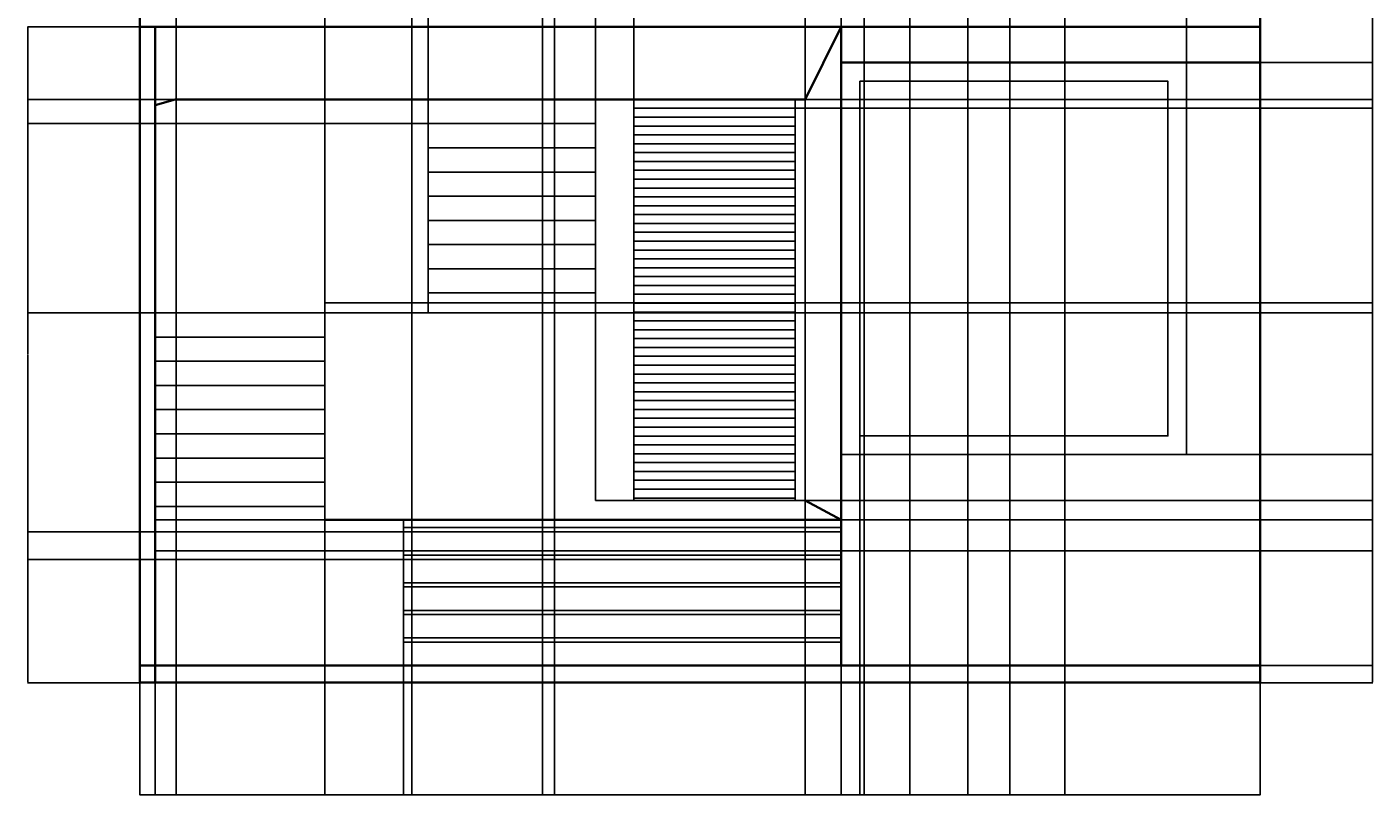
# Model space of a CAD drawing. Units: feet. Extents: x 2373 to 3800, y 799 to 1842.
# Tile 2 of 4: x 3224 to 3800, y 799 to 1129. Entities that reach past the tile are written whole.
import ezdxf

# ---------------------------------------------------------------- set-up
doc = ezdxf.new("R2010")
doc.units = ezdxf.units.FT
for name, color, linetype, lineweight in [('A-ANNO-DIMS', 2, 'Continuous', 18), ('A-DOOR', 4, 'Continuous', 25), ('A-ELEV', 7, 'Continuous', 35), ('A-FLOR-STRS', 3, 'Continuous', 25), ('A-GLAZ', 4, 'Continuous', 25)]:
    doc.layers.add(name, color=color, linetype=linetype, lineweight=lineweight)
doc.styles.get("Standard").update_dxf_attribs({"font": 'arial.ttf'})
doc.dimstyles.get("Standard").update_dxf_attribs({"dimtxt": 0.18, "dimasz": 0.18, "dimexe": 0.18, "dimexo": 0.0625, "dimgap": 0.09, "dimtad": 0, "dimtih": 1, "dimtoh": 1, "dimdec": 1, "dimzin": 0, "dimdsep": 46, "dimlunit": 3, "dimtxsty": 'Standard', "dimcen": 0.09, "dimadec": 0, "dimazin": 0, "dimtfac": 1, "dimtdec": 1, "dimtofl": 0, "dimtmove": 0, "dimatfit": 3, "dimfxl": 1, "dimtolj": 1, "dimtzin": 0, "dimarcsym": 0})

# ---------------------------------------------------------------- blocks, each defined once
blk = doc.blocks.new('*D7')
at = {"layer": 'A-ANNO-DIMS', "color": 0, "lineweight": -2, "transparency": 16777216}
for p, q in [((3271.99, 847.59), (3271.99, 799.47)), ((3751.99, 847.59), (3751.99, 799.47)), ((3272.17, 799.65), (3511.69, 799.65)), ((3751.81, 799.65), (3512.28, 799.65))]:
    blk.add_line(p, q, dxfattribs=at)
at = {"layer": 'A-ANNO-DIMS', "color": 0, "transparency": 16777216}
for points in [[(3272.17, 799.68), (3272.17, 799.62), (3271.99, 799.65)], [(3751.81, 799.68), (3751.81, 799.62), (3751.99, 799.65)]]:
    blk.add_solid(points, dxfattribs=at)
at = {"layer": 'Defpoints', "color": 0, "transparency": 16777216}
for p in [(3271.99, 847.65), (3751.99, 847.65), (3751.99, 799.65)]:
    blk.add_point(p, dxfattribs=at)
at = {"layer": 'A-ANNO-DIMS', "color": 0, "transparency": 16777216, "insert": (3511.99, 799.65), "char_height": 0.18, "attachment_point": 5}
blk.add_mtext('\\A1;480', dxfattribs=at)
blk = doc.blocks.new('*D8')
at = {"layer": 'A-ANNO-DIMS', "color": 0, "lineweight": -2, "transparency": 16777216}
for p, q in [((3752.05, 1793.54), (3800.17, 1793.54)), ((3799.99, 1793.36), (3799.99, 1320.78)), ((3799.99, 847.83), (3799.99, 1320.41)), ((3752.05, 847.65), (3800.17, 847.65))]:
    blk.add_line(p, q, dxfattribs=at)
at = {"layer": 'A-ANNO-DIMS', "color": 0, "transparency": 16777216}
for points in [[(3799.96, 1793.36), (3800.02, 1793.36), (3799.99, 1793.54)], [(3799.96, 847.83), (3800.02, 847.83), (3799.99, 847.65)]]:
    blk.add_solid(points, dxfattribs=at)
at = {"layer": 'Defpoints', "color": 0, "transparency": 16777216}
for p in [(3751.99, 1793.54), (3799.99, 1793.54), (3751.99, 847.65)]:
    blk.add_point(p, dxfattribs=at)
at = {"layer": 'A-ANNO-DIMS', "color": 0, "transparency": 16777216, "insert": (3799.99, 1320.6), "char_height": 0.18, "attachment_point": 5}
blk.add_mtext('\\A1;945.9', dxfattribs=at)
blk = doc.blocks.new('*D9')
at = {"layer": 'A-ANNO-DIMS', "color": 0, "lineweight": -2, "transparency": 16777216}
for p, q in [((3271.92, 1128.67), (3223.81, 1128.67)), ((3223.99, 1128.49), (3223.99, 988.34)), ((3223.99, 847.83), (3223.99, 987.98)), ((3271.92, 847.65), (3223.81, 847.65))]:
    blk.add_line(p, q, dxfattribs=at)
at = {"layer": 'A-ANNO-DIMS', "color": 0, "transparency": 16777216}
for points in [[(3223.96, 1128.49), (3224.02, 1128.49), (3223.99, 1128.67)], [(3223.96, 847.83), (3224.02, 847.83), (3223.99, 847.65)]]:
    blk.add_solid(points, dxfattribs=at)
at = {"layer": 'Defpoints', "color": 0, "transparency": 16777216}
for p in [(3223.99, 1128.67), (3271.99, 1128.67), (3271.99, 847.65)]:
    blk.add_point(p, dxfattribs=at)
at = {"layer": 'A-ANNO-DIMS', "color": 0, "transparency": 16777216, "insert": (3223.99, 988.16), "char_height": 0.18, "attachment_point": 5}
blk.add_mtext('\\A1;281', dxfattribs=at)
blk = doc.blocks.new('*D18')
at = {"layer": 'A-ANNO-DIMS', "color": 0, "lineweight": -2, "transparency": 16777216}
for p, q in [((3271.99, 854.9), (3271.99, 799.47)), ((3384.96, 854.9), (3384.96, 799.47)), ((3272.17, 799.65), (3328.02, 799.65)), ((3384.78, 799.65), (3328.93, 799.65))]:
    blk.add_line(p, q, dxfattribs=at)
at = {"layer": 'A-ANNO-DIMS', "color": 0, "transparency": 16777216}
for points in [[(3272.17, 799.68), (3272.17, 799.62), (3271.99, 799.65)], [(3384.78, 799.68), (3384.78, 799.62), (3384.96, 799.65)]]:
    blk.add_solid(points, dxfattribs=at)
at = {"layer": 'Defpoints', "color": 0, "transparency": 16777216}
for p in [(3271.99, 854.96), (3384.96, 854.96), (3384.96, 799.65)]:
    blk.add_point(p, dxfattribs=at)
at = {"layer": 'A-ANNO-DIMS', "color": 0, "transparency": 16777216, "insert": (3328.47, 799.65), "char_height": 0.18, "attachment_point": 5}
blk.add_mtext('\\A1;112.98', dxfattribs=at)
blk = doc.blocks.new('*D19')
at = {"layer": 'A-ANNO-DIMS', "color": 0, "lineweight": -2, "transparency": 16777216}
for p, q in [((3572.43, 917.3), (3572.43, 799.47)), ((3384.96, 854.9), (3384.96, 799.47)), ((3385.14, 799.65), (3478.24, 799.65)), ((3572.25, 799.65), (3479.15, 799.65))]:
    blk.add_line(p, q, dxfattribs=at)
at = {"layer": 'A-ANNO-DIMS', "color": 0, "transparency": 16777216}
for points in [[(3385.14, 799.68), (3385.14, 799.62), (3384.96, 799.65)], [(3572.25, 799.68), (3572.25, 799.62), (3572.43, 799.65)]]:
    blk.add_solid(points, dxfattribs=at)
at = {"layer": 'Defpoints', "color": 0, "transparency": 16777216}
for p in [(3572.43, 917.36), (3384.96, 854.96), (3572.43, 799.65)]:
    blk.add_point(p, dxfattribs=at)
at = {"layer": 'A-ANNO-DIMS', "color": 0, "transparency": 16777216, "insert": (3478.7, 799.65), "char_height": 0.18, "attachment_point": 5}
blk.add_mtext('\\A1;187.47', dxfattribs=at)
blk = doc.blocks.new('*D20')
at = {"layer": 'A-ANNO-DIMS', "color": 0, "lineweight": -2, "transparency": 16777216}
for p, q in [((3572.43, 945.53), (3572.43, 1841.72)), ((3572.61, 1841.54), (3645.95, 1841.54)), ((3720.2, 1841.54), (3646.87, 1841.54)), ((3720.38, 1113.42), (3720.38, 1841.72))]:
    blk.add_line(p, q, dxfattribs=at)
at = {"layer": 'A-ANNO-DIMS', "color": 0, "transparency": 16777216}
for points in [[(3572.61, 1841.57), (3572.61, 1841.51), (3572.43, 1841.54)], [(3720.2, 1841.57), (3720.2, 1841.51), (3720.38, 1841.54)]]:
    blk.add_solid(points, dxfattribs=at)
at = {"layer": 'Defpoints', "color": 0, "transparency": 16777216}
for p in [(3720.38, 1841.54), (3720.38, 1113.36), (3572.43, 945.46)]:
    blk.add_point(p, dxfattribs=at)
at = {"layer": 'A-ANNO-DIMS', "color": 0, "transparency": 16777216, "insert": (3646.41, 1841.54), "char_height": 0.18, "attachment_point": 5}
blk.add_mtext('\\A1;147.95', dxfattribs=at)
blk = doc.blocks.new('*D21')
at = {"layer": 'A-ANNO-DIMS', "color": 0, "lineweight": -2, "transparency": 16777216}
for p, q in [((3720.45, 1113.36), (3800.17, 1113.36)), ((3799.99, 1113.18), (3799.99, 1029.59)), ((3799.99, 945.64), (3799.99, 1029.23)), ((3720.45, 945.46), (3800.17, 945.46))]:
    blk.add_line(p, q, dxfattribs=at)
at = {"layer": 'A-ANNO-DIMS', "color": 0, "transparency": 16777216}
for points in [[(3799.96, 1113.18), (3800.02, 1113.18), (3799.99, 1113.36)], [(3799.96, 945.64), (3800.02, 945.64), (3799.99, 945.46)]]:
    blk.add_solid(points, dxfattribs=at)
at = {"layer": 'Defpoints', "color": 0, "transparency": 16777216}
for p in [(3720.38, 1113.36), (3799.99, 1113.36), (3720.38, 945.46)]:
    blk.add_point(p, dxfattribs=at)
at = {"layer": 'A-ANNO-DIMS', "color": 0, "transparency": 16777216, "insert": (3799.99, 1029.41), "char_height": 0.18, "attachment_point": 5}
blk.add_mtext('\\A1;167.9', dxfattribs=at)
blk = doc.blocks.new('*D22')
at = {"layer": 'A-ANNO-DIMS', "color": 0, "lineweight": -2, "transparency": 16777216}
for p, q in [((3720.45, 945.46), (3800.17, 945.46)), ((3799.99, 945.28), (3799.99, 896.74)), ((3799.99, 847.83), (3799.99, 896.38)), ((3752.05, 847.65), (3800.17, 847.65))]:
    blk.add_line(p, q, dxfattribs=at)
at = {"layer": 'A-ANNO-DIMS', "color": 0, "transparency": 16777216}
for points in [[(3799.96, 945.28), (3800.02, 945.28), (3799.99, 945.46)], [(3799.96, 847.83), (3800.02, 847.83), (3799.99, 847.65)]]:
    blk.add_solid(points, dxfattribs=at)
at = {"layer": 'Defpoints', "color": 0, "transparency": 16777216}
for p in [(3720.38, 945.46), (3799.99, 945.46), (3751.99, 847.65)]:
    blk.add_point(p, dxfattribs=at)
at = {"layer": 'A-ANNO-DIMS', "color": 0, "transparency": 16777216, "insert": (3799.99, 896.56), "char_height": 0.18, "attachment_point": 5}
blk.add_mtext('\\A1;97.81', dxfattribs=at)
blk = doc.blocks.new('*D23')
at = {"layer": 'A-ANNO-DIMS', "color": 0, "lineweight": -2, "transparency": 16777216}
for p, q in [((3483.65, 925.75), (3483.65, 1841.72)), ((3483.83, 1841.54), (3519.95, 1841.54)), ((3556.84, 1841.54), (3520.73, 1841.54)), ((3557.02, 1097.65), (3557.02, 1841.72))]:
    blk.add_line(p, q, dxfattribs=at)
at = {"layer": 'A-ANNO-DIMS', "color": 0, "transparency": 16777216}
for points in [[(3483.83, 1841.57), (3483.83, 1841.51), (3483.65, 1841.54)], [(3556.84, 1841.57), (3556.84, 1841.51), (3557.02, 1841.54)]]:
    blk.add_solid(points, dxfattribs=at)
at = {"layer": 'Defpoints', "color": 0, "transparency": 16777216}
for p in [(3557.02, 1841.54), (3557.02, 1097.59), (3483.65, 925.69)]:
    blk.add_point(p, dxfattribs=at)
at = {"layer": 'A-ANNO-DIMS', "color": 0, "transparency": 16777216, "insert": (3520.34, 1841.54), "char_height": 0.18, "attachment_point": 5}
blk.add_mtext('\\A1;73.37', dxfattribs=at)
blk = doc.blocks.new('*D24')
at = {"layer": 'A-ANNO-DIMS', "color": 0, "lineweight": -2, "transparency": 16777216}
for p, q in [((3557.09, 1097.59), (3800.17, 1097.59)), ((3799.99, 1097.41), (3799.99, 1011.82)), ((3799.99, 925.87), (3799.99, 1011.46)), ((3557.09, 925.69), (3800.17, 925.69))]:
    blk.add_line(p, q, dxfattribs=at)
at = {"layer": 'A-ANNO-DIMS', "color": 0, "transparency": 16777216}
for points in [[(3799.96, 1097.41), (3800.02, 1097.41), (3799.99, 1097.59)], [(3799.96, 925.87), (3800.02, 925.87), (3799.99, 925.69)]]:
    blk.add_solid(points, dxfattribs=at)
at = {"layer": 'Defpoints', "color": 0, "transparency": 16777216}
for p in [(3557.02, 1097.59), (3799.99, 1097.59), (3557.02, 925.69)]:
    blk.add_point(p, dxfattribs=at)
at = {"layer": 'A-ANNO-DIMS', "color": 0, "transparency": 16777216, "insert": (3799.99, 1011.64), "char_height": 0.18, "attachment_point": 5}
blk.add_mtext('\\A1;171.9', dxfattribs=at)
blk = doc.blocks.new('*D27')
at = {"layer": 'A-ANNO-DIMS', "color": 0, "lineweight": -2, "transparency": 16777216}
for p, q in [((3444.52, 1624.82), (3444.52, 799.47)), ((3449.58, 1616.05), (3449.58, 799.47)), ((3444.7, 799.65), (3446.65, 799.65)), ((3449.4, 799.65), (3447.44, 799.65))]:
    blk.add_line(p, q, dxfattribs=at)
at = {"layer": 'A-ANNO-DIMS', "color": 0, "transparency": 16777216}
for points in [[(3444.7, 799.68), (3444.7, 799.62), (3444.52, 799.65)], [(3449.4, 799.68), (3449.4, 799.62), (3449.58, 799.65)]]:
    blk.add_solid(points, dxfattribs=at)
at = {"layer": 'Defpoints', "color": 0, "transparency": 16777216}
for p in [(3444.52, 1624.88), (3449.58, 1616.11), (3449.58, 799.65)]:
    blk.add_point(p, dxfattribs=at)
at = {"layer": 'A-ANNO-DIMS', "color": 0, "transparency": 16777216, "insert": (3447.05, 799.65), "char_height": 0.18, "attachment_point": 5}
blk.add_mtext('\\A1;5.057', dxfattribs=at)
blk = doc.blocks.new('*D28')
at = {"layer": 'A-ANNO-DIMS', "color": 0, "lineweight": -2, "transparency": 16777216}
for p, q in [((3271.99, 1380.79), (3271.99, 799.47)), ((3388.52, 1380.79), (3388.52, 799.47)), ((3272.17, 799.65), (3329.8, 799.65)), ((3388.34, 799.65), (3330.71, 799.65))]:
    blk.add_line(p, q, dxfattribs=at)
at = {"layer": 'A-ANNO-DIMS', "color": 0, "transparency": 16777216}
for points in [[(3272.17, 799.68), (3272.17, 799.62), (3271.99, 799.65)], [(3388.34, 799.68), (3388.34, 799.62), (3388.52, 799.65)]]:
    blk.add_solid(points, dxfattribs=at)
at = {"layer": 'Defpoints', "color": 0, "transparency": 16777216}
for p in [(3271.99, 1380.85), (3388.52, 1380.85), (3388.52, 799.65)]:
    blk.add_point(p, dxfattribs=at)
at = {"layer": 'A-ANNO-DIMS', "color": 0, "transparency": 16777216, "insert": (3330.25, 799.65), "char_height": 0.18, "attachment_point": 5}
blk.add_mtext('\\A1;116.53', dxfattribs=at)
blk = doc.blocks.new('*D30')
at = {"layer": 'A-ANNO-DIMS', "color": 0, "lineweight": -2, "transparency": 16777216}
for p, q in [((3271.99, 1366.11), (3271.99, 799.47)), ((3287.49, 1366.11), (3287.49, 799.47)), ((3272.17, 799.65), (3279.42, 799.65)), ((3287.31, 799.65), (3280.05, 799.65))]:
    blk.add_line(p, q, dxfattribs=at)
at = {"layer": 'A-ANNO-DIMS', "color": 0, "transparency": 16777216}
for points in [[(3272.17, 799.68), (3272.17, 799.62), (3271.99, 799.65)], [(3287.31, 799.68), (3287.31, 799.62), (3287.49, 799.65)]]:
    blk.add_solid(points, dxfattribs=at)
at = {"layer": 'Defpoints', "color": 0, "transparency": 16777216}
for p in [(3271.99, 1366.18), (3287.49, 1366.18), (3287.49, 799.65)]:
    blk.add_point(p, dxfattribs=at)
at = {"layer": 'A-ANNO-DIMS', "color": 0, "transparency": 16777216, "insert": (3279.74, 799.65), "char_height": 0.18, "attachment_point": 5}
blk.add_mtext('\\A1;15.5', dxfattribs=at)
blk = doc.blocks.new('*D32')
at = {"layer": 'A-ANNO-DIMS', "color": 0, "lineweight": -2, "transparency": 16777216}
for p, q in [((3278.6, 904.12), (3278.6, 799.47)), ((3351.18, 904.12), (3351.18, 799.47)), ((3278.78, 799.65), (3314.5, 799.65)), ((3351, 799.65), (3315.28, 799.65))]:
    blk.add_line(p, q, dxfattribs=at)
at = {"layer": 'A-ANNO-DIMS', "color": 0, "transparency": 16777216}
for points in [[(3278.78, 799.68), (3278.78, 799.62), (3278.6, 799.65)], [(3351, 799.68), (3351, 799.62), (3351.18, 799.65)]]:
    blk.add_solid(points, dxfattribs=at)
at = {"layer": 'Defpoints', "color": 0, "transparency": 16777216}
for p in [(3278.6, 904.18), (3351.18, 904.18), (3351.18, 799.65)]:
    blk.add_point(p, dxfattribs=at)
at = {"layer": 'A-ANNO-DIMS', "color": 0, "transparency": 16777216, "insert": (3314.89, 799.65), "char_height": 0.18, "attachment_point": 5}
blk.add_mtext('\\A1;72.57', dxfattribs=at)
blk = doc.blocks.new('*D33')
at = {"layer": 'A-ANNO-DIMS', "color": 0, "lineweight": -2, "transparency": 16777216}
for p, q in [((3351.24, 917.36), (3800.17, 917.36)), ((3799.99, 917.18), (3799.99, 910.95)), ((3799.99, 904.36), (3799.99, 910.59)), ((3351.24, 904.18), (3800.17, 904.18))]:
    blk.add_line(p, q, dxfattribs=at)
at = {"layer": 'A-ANNO-DIMS', "color": 0, "transparency": 16777216}
for points in [[(3799.96, 917.18), (3800.02, 917.18), (3799.99, 917.36)], [(3799.96, 904.36), (3800.02, 904.36), (3799.99, 904.18)]]:
    blk.add_solid(points, dxfattribs=at)
at = {"layer": 'Defpoints', "color": 0, "transparency": 16777216}
for p in [(3351.18, 917.36), (3799.99, 917.36), (3351.18, 904.18)]:
    blk.add_point(p, dxfattribs=at)
at = {"layer": 'A-ANNO-DIMS', "color": 0, "transparency": 16777216, "insert": (3799.99, 910.77), "char_height": 0.18, "attachment_point": 5}
blk.add_mtext('\\A1;13.18', dxfattribs=at)
blk = doc.blocks.new('*D34')
at = {"layer": 'A-ANNO-DIMS', "color": 0, "lineweight": -2, "transparency": 16777216}
for p, q in [((3351.24, 1006.12), (3800.17, 1006.12)), ((3799.99, 1005.94), (3799.99, 961.92)), ((3799.99, 917.54), (3799.99, 961.56)), ((3351.24, 917.36), (3800.17, 917.36))]:
    blk.add_line(p, q, dxfattribs=at)
at = {"layer": 'A-ANNO-DIMS', "color": 0, "transparency": 16777216}
for points in [[(3799.96, 1005.94), (3800.02, 1005.94), (3799.99, 1006.12)], [(3799.96, 917.54), (3800.02, 917.54), (3799.99, 917.36)]]:
    blk.add_solid(points, dxfattribs=at)
at = {"layer": 'Defpoints', "color": 0, "transparency": 16777216}
for p in [(3351.18, 1006.12), (3799.99, 1006.12), (3351.18, 917.36)]:
    blk.add_point(p, dxfattribs=at)
at = {"layer": 'A-ANNO-DIMS', "color": 0, "transparency": 16777216, "insert": (3799.99, 961.74), "char_height": 0.18, "attachment_point": 5}
blk.add_mtext('\\A1;88.76', dxfattribs=at)
blk = doc.blocks.new('*D35')
at = {"layer": 'A-ANNO-DIMS', "color": 0, "lineweight": -2, "transparency": 16777216}
for p, q in [((3351.24, 1010.41), (3800.17, 1010.41)), ((3799.99, 1010.23), (3799.99, 1008.45)), ((3351.24, 1006.12), (3800.17, 1006.12)), ((3799.99, 1006.3), (3799.99, 1008.08))]:
    blk.add_line(p, q, dxfattribs=at)
at = {"layer": 'A-ANNO-DIMS', "color": 0, "transparency": 16777216}
for points in [[(3799.96, 1010.23), (3800.02, 1010.23), (3799.99, 1010.41)], [(3799.96, 1006.3), (3800.02, 1006.3), (3799.99, 1006.12)]]:
    blk.add_solid(points, dxfattribs=at)
at = {"layer": 'Defpoints', "color": 0, "transparency": 16777216}
for p in [(3351.18, 1010.41), (3799.99, 1010.41), (3351.18, 1006.12)]:
    blk.add_point(p, dxfattribs=at)
at = {"layer": 'A-ANNO-DIMS', "color": 0, "transparency": 16777216, "insert": (3799.99, 1008.27), "char_height": 0.18, "attachment_point": 5}
blk.add_mtext('\\A1;4.295', dxfattribs=at)
blk = doc.blocks.new('*D36')
at = {"layer": 'A-ANNO-DIMS', "color": 0, "lineweight": -2, "transparency": 16777216}
for p, q in [((3351.18, 1010.48), (3351.18, 1841.72)), ((3351.36, 1841.54), (3372.95, 1841.54)), ((3395.3, 1841.54), (3373.71, 1841.54)), ((3395.48, 1010.48), (3395.48, 1841.72))]:
    blk.add_line(p, q, dxfattribs=at)
at = {"layer": 'A-ANNO-DIMS', "color": 0, "transparency": 16777216}
for points in [[(3351.36, 1841.57), (3351.36, 1841.51), (3351.18, 1841.54)], [(3395.3, 1841.57), (3395.3, 1841.51), (3395.48, 1841.54)]]:
    blk.add_solid(points, dxfattribs=at)
at = {"layer": 'Defpoints', "color": 0, "transparency": 16777216}
for p in [(3395.48, 1841.54), (3351.18, 1010.41), (3395.48, 1010.41)]:
    blk.add_point(p, dxfattribs=at)
at = {"layer": 'A-ANNO-DIMS', "color": 0, "transparency": 16777216, "insert": (3373.33, 1841.54), "char_height": 0.18, "attachment_point": 5}
blk.add_mtext('\\A1;44.31', dxfattribs=at)
blk = doc.blocks.new('*D37')
at = {"layer": 'A-ANNO-DIMS', "color": 0, "lineweight": -2, "transparency": 16777216}
for p, q in [((3395.48, 1097.65), (3395.48, 1841.72)), ((3395.66, 1841.54), (3430.91, 1841.54)), ((3466.94, 1841.54), (3431.69, 1841.54)), ((3467.12, 1097.65), (3467.12, 1841.72))]:
    blk.add_line(p, q, dxfattribs=at)
at = {"layer": 'A-ANNO-DIMS', "color": 0, "transparency": 16777216}
for points in [[(3395.66, 1841.57), (3395.66, 1841.51), (3395.48, 1841.54)], [(3466.94, 1841.57), (3466.94, 1841.51), (3467.12, 1841.54)]]:
    blk.add_solid(points, dxfattribs=at)
at = {"layer": 'Defpoints', "color": 0, "transparency": 16777216}
for p in [(3467.12, 1841.54), (3395.48, 1097.59), (3467.12, 1097.59)]:
    blk.add_point(p, dxfattribs=at)
at = {"layer": 'A-ANNO-DIMS', "color": 0, "transparency": 16777216, "insert": (3431.3, 1841.54), "char_height": 0.18, "attachment_point": 5}
blk.add_mtext('\\A1;71.63', dxfattribs=at)
blk = doc.blocks.new('*D38')
at = {"layer": 'A-ANNO-DIMS', "color": 0, "lineweight": -2, "transparency": 16777216}
for p, q in [((3467.12, 1097.65), (3467.12, 1841.72)), ((3467.3, 1841.54), (3474.93, 1841.54)), ((3483.47, 1841.54), (3475.84, 1841.54)), ((3483.65, 1097.65), (3483.65, 1841.72))]:
    blk.add_line(p, q, dxfattribs=at)
at = {"layer": 'A-ANNO-DIMS', "color": 0, "transparency": 16777216}
for points in [[(3467.3, 1841.57), (3467.3, 1841.51), (3467.12, 1841.54)], [(3483.47, 1841.57), (3483.47, 1841.51), (3483.65, 1841.54)]]:
    blk.add_solid(points, dxfattribs=at)
at = {"layer": 'Defpoints', "color": 0, "transparency": 16777216}
for p in [(3483.65, 1841.54), (3467.12, 1097.59), (3483.65, 1097.59)]:
    blk.add_point(p, dxfattribs=at)
at = {"layer": 'A-ANNO-DIMS', "color": 0, "transparency": 16777216, "insert": (3475.39, 1841.54), "char_height": 0.18, "attachment_point": 5}
blk.add_mtext('\\A1;16.537', dxfattribs=at)
blk = doc.blocks.new('*D39')
at = {"layer": 'A-ANNO-DIMS', "color": 0, "lineweight": -2, "transparency": 16777216}
for p, q in [((3395.42, 1097.59), (3223.81, 1097.59)), ((3223.99, 1097.41), (3223.99, 1052.03)), ((3223.99, 1006.3), (3223.99, 1051.67)), ((3395.42, 1006.12), (3223.81, 1006.12))]:
    blk.add_line(p, q, dxfattribs=at)
at = {"layer": 'A-ANNO-DIMS', "color": 0, "transparency": 16777216}
for points in [[(3223.96, 1097.41), (3224.02, 1097.41), (3223.99, 1097.59)], [(3223.96, 1006.3), (3224.02, 1006.3), (3223.99, 1006.12)]]:
    blk.add_solid(points, dxfattribs=at)
at = {"layer": 'Defpoints', "color": 0, "transparency": 16777216}
for p in [(3223.99, 1097.59), (3395.48, 1097.59), (3395.48, 1006.12)]:
    blk.add_point(p, dxfattribs=at)
at = {"layer": 'A-ANNO-DIMS', "color": 0, "transparency": 16777216, "insert": (3223.99, 1051.85), "char_height": 0.18, "attachment_point": 5}
blk.add_mtext('\\A1;91.47', dxfattribs=at)
blk = doc.blocks.new('*D40')
at = {"layer": 'A-ANNO-DIMS', "color": 0, "lineweight": -2, "transparency": 16777216}
for p, q in [((3395.42, 1097.59), (3223.81, 1097.59)), ((3223.99, 1097.41), (3223.99, 1092.58)), ((3223.99, 1087.4), (3223.99, 1092.22)), ((3395.42, 1087.22), (3223.81, 1087.22))]:
    blk.add_line(p, q, dxfattribs=at)
at = {"layer": 'A-ANNO-DIMS', "color": 0, "transparency": 16777216}
for points in [[(3223.96, 1097.41), (3224.02, 1097.41), (3223.99, 1097.59)], [(3223.96, 1087.4), (3224.02, 1087.4), (3223.99, 1087.22)]]:
    blk.add_solid(points, dxfattribs=at)
at = {"layer": 'Defpoints', "color": 0, "transparency": 16777216}
for p in [(3223.99, 1097.59), (3395.48, 1097.59), (3395.48, 1087.22)]:
    blk.add_point(p, dxfattribs=at)
at = {"layer": 'A-ANNO-DIMS', "color": 0, "transparency": 16777216, "insert": (3223.99, 1092.4), "char_height": 0.18, "attachment_point": 5}
blk.add_mtext('\\A1;10.368', dxfattribs=at)
blk = doc.blocks.new('*D41')
at = {"layer": 'A-ANNO-DIMS', "color": 0, "lineweight": -2, "transparency": 16777216}
for p, q in [((3384.9, 912.34), (3223.81, 912.34)), ((3223.99, 912.16), (3223.99, 906.6)), ((3223.99, 900.68), (3223.99, 906.24)), ((3384.9, 900.5), (3223.81, 900.5))]:
    blk.add_line(p, q, dxfattribs=at)
at = {"layer": 'A-ANNO-DIMS', "color": 0, "transparency": 16777216}
for points in [[(3223.96, 912.16), (3224.02, 912.16), (3223.99, 912.34)], [(3223.96, 900.68), (3224.02, 900.68), (3223.99, 900.5)]]:
    blk.add_solid(points, dxfattribs=at)
at = {"layer": 'Defpoints', "color": 0, "transparency": 16777216}
for p in [(3223.99, 912.34), (3384.96, 912.34), (3384.96, 900.5)]:
    blk.add_point(p, dxfattribs=at)
at = {"layer": 'A-ANNO-DIMS', "color": 0, "transparency": 16777216, "insert": (3223.99, 906.42), "char_height": 0.18, "attachment_point": 5}
blk.add_mtext('\\A1;11.837', dxfattribs=at)
blk = doc.blocks.new('*D42')
at = {"layer": 'A-ANNO-DIMS', "color": 0, "lineweight": -2, "transparency": 16777216}
for p, q in [((3572.5, 917.36), (3800.17, 917.36)), ((3799.99, 917.18), (3799.99, 886.34)), ((3799.99, 855.14), (3799.99, 885.98)), ((3572.5, 854.96), (3800.17, 854.96))]:
    blk.add_line(p, q, dxfattribs=at)
at = {"layer": 'A-ANNO-DIMS', "color": 0, "transparency": 16777216}
for points in [[(3799.96, 917.18), (3800.02, 917.18), (3799.99, 917.36)], [(3799.96, 855.14), (3800.02, 855.14), (3799.99, 854.96)]]:
    blk.add_solid(points, dxfattribs=at)
at = {"layer": 'Defpoints', "color": 0, "transparency": 16777216}
for p in [(3572.43, 917.36), (3799.99, 917.36), (3572.43, 854.96)]:
    blk.add_point(p, dxfattribs=at)
at = {"layer": 'A-ANNO-DIMS', "color": 0, "transparency": 16777216, "insert": (3799.99, 886.16), "char_height": 0.18, "attachment_point": 5}
blk.add_mtext('\\A1;62.4', dxfattribs=at)
blk = doc.blocks.new('*D43')
at = {"layer": 'A-ANNO-DIMS', "color": 0, "lineweight": -2, "transparency": 16777216}
for p, q in [((3557.09, 925.69), (3800.17, 925.69)), ((3799.99, 925.51), (3799.99, 921.71)), ((3572.5, 917.36), (3800.17, 917.36)), ((3799.99, 917.54), (3799.99, 921.34))]:
    blk.add_line(p, q, dxfattribs=at)
at = {"layer": 'A-ANNO-DIMS', "color": 0, "transparency": 16777216}
for points in [[(3799.96, 925.51), (3800.02, 925.51), (3799.99, 925.69)], [(3799.96, 917.54), (3800.02, 917.54), (3799.99, 917.36)]]:
    blk.add_solid(points, dxfattribs=at)
at = {"layer": 'Defpoints', "color": 0, "transparency": 16777216}
for p in [(3557.02, 925.69), (3799.99, 925.69), (3572.43, 917.36)]:
    blk.add_point(p, dxfattribs=at)
at = {"layer": 'A-ANNO-DIMS', "color": 0, "transparency": 16777216, "insert": (3799.99, 921.52), "char_height": 0.18, "attachment_point": 5}
blk.add_mtext('\\A1;8.327', dxfattribs=at)
blk = doc.blocks.new('*D44')
at = {"layer": 'A-ANNO-DIMS', "color": 0, "lineweight": -2, "transparency": 16777216}
for p, q in [((3557.02, 925.62), (3557.02, 799.47)), ((3572.43, 917.3), (3572.43, 799.47)), ((3557.2, 799.65), (3564.36, 799.65)), ((3572.25, 799.65), (3565.1, 799.65))]:
    blk.add_line(p, q, dxfattribs=at)
at = {"layer": 'A-ANNO-DIMS', "color": 0, "transparency": 16777216}
for points in [[(3557.2, 799.68), (3557.2, 799.62), (3557.02, 799.65)], [(3572.25, 799.68), (3572.25, 799.62), (3572.43, 799.65)]]:
    blk.add_solid(points, dxfattribs=at)
at = {"layer": 'Defpoints', "color": 0, "transparency": 16777216}
for p in [(3557.02, 925.69), (3572.43, 917.36), (3572.43, 799.65)]:
    blk.add_point(p, dxfattribs=at)
at = {"layer": 'A-ANNO-DIMS', "color": 0, "transparency": 16777216, "insert": (3564.73, 799.65), "char_height": 0.18, "attachment_point": 5}
blk.add_mtext('\\A1;15.41', dxfattribs=at)
blk = doc.blocks.new('*D45')
at = {"layer": 'A-ANNO-DIMS', "color": 0, "lineweight": -2, "transparency": 16777216}
for p, q in [((3552.81, 1097.59), (3800.17, 1097.59)), ((3799.99, 1097.41), (3799.99, 1095.87)), ((3552.81, 1093.79), (3800.17, 1093.79)), ((3799.99, 1093.97), (3799.99, 1095.51))]:
    blk.add_line(p, q, dxfattribs=at)
at = {"layer": 'A-ANNO-DIMS', "color": 0, "transparency": 16777216}
for points in [[(3799.96, 1097.41), (3800.02, 1097.41), (3799.99, 1097.59)], [(3799.96, 1093.97), (3800.02, 1093.97), (3799.99, 1093.79)]]:
    blk.add_solid(points, dxfattribs=at)
at = {"layer": 'Defpoints', "color": 0, "transparency": 16777216}
for p in [(3552.74, 1097.59), (3799.99, 1097.59), (3552.74, 1093.79)]:
    blk.add_point(p, dxfattribs=at)
at = {"layer": 'A-ANNO-DIMS', "color": 0, "transparency": 16777216, "insert": (3799.99, 1095.69), "char_height": 0.18, "attachment_point": 5}
blk.add_mtext('\\A1;3.796', dxfattribs=at)
blk = doc.blocks.new('*D46')
at = {"layer": 'A-ANNO-DIMS', "color": 0, "lineweight": -2, "transparency": 16777216}
for p, q in [((3580.39, 953.36), (3580.39, 799.47)), ((3572.43, 945.4), (3572.43, 799.47)), ((3572.61, 799.65), (3576.02, 799.65)), ((3580.21, 799.65), (3576.8, 799.65))]:
    blk.add_line(p, q, dxfattribs=at)
at = {"layer": 'A-ANNO-DIMS', "color": 0, "transparency": 16777216}
for points in [[(3572.61, 799.68), (3572.61, 799.62), (3572.43, 799.65)], [(3580.21, 799.68), (3580.21, 799.62), (3580.39, 799.65)]]:
    blk.add_solid(points, dxfattribs=at)
at = {"layer": 'Defpoints', "color": 0, "transparency": 16777216}
for p in [(3580.39, 953.42), (3572.43, 945.46), (3580.39, 799.65)]:
    blk.add_point(p, dxfattribs=at)
at = {"layer": 'A-ANNO-DIMS', "color": 0, "transparency": 16777216, "insert": (3576.41, 799.65), "char_height": 0.18, "attachment_point": 5}
blk.add_mtext('\\A1;7.953', dxfattribs=at)
blk = doc.blocks.new('*D48')
at = {"layer": 'A-ANNO-DIMS', "color": 0, "lineweight": -2, "transparency": 16777216}
for p, q in [((3582.33, 1693.47), (3582.33, 799.47)), ((3601.88, 1658.52), (3601.88, 799.47)), ((3582.51, 799.65), (3591.72, 799.65)), ((3601.7, 799.65), (3592.49, 799.65))]:
    blk.add_line(p, q, dxfattribs=at)
at = {"layer": 'A-ANNO-DIMS', "color": 0, "transparency": 16777216}
for points in [[(3582.51, 799.68), (3582.51, 799.62), (3582.33, 799.65)], [(3601.7, 799.68), (3601.7, 799.62), (3601.88, 799.65)]]:
    blk.add_solid(points, dxfattribs=at)
at = {"layer": 'Defpoints', "color": 0, "transparency": 16777216}
for p in [(3582.33, 1693.53), (3601.88, 1658.58), (3601.88, 799.65)]:
    blk.add_point(p, dxfattribs=at)
at = {"layer": 'A-ANNO-DIMS', "color": 0, "transparency": 16777216, "insert": (3592.11, 799.65), "char_height": 0.18, "attachment_point": 5}
blk.add_mtext('\\A1;19.55', dxfattribs=at)
blk = doc.blocks.new('*D49')
at = {"layer": 'A-ANNO-DIMS', "color": 0, "lineweight": -2, "transparency": 16777216}
for p, q in [((3626.67, 1690.12), (3626.67, 799.47)), ((3601.88, 1658.52), (3601.88, 799.47)), ((3602.06, 799.65), (3613.88, 799.65)), ((3626.49, 799.65), (3614.67, 799.65))]:
    blk.add_line(p, q, dxfattribs=at)
at = {"layer": 'A-ANNO-DIMS', "color": 0, "transparency": 16777216}
for points in [[(3602.06, 799.68), (3602.06, 799.62), (3601.88, 799.65)], [(3626.49, 799.68), (3626.49, 799.62), (3626.67, 799.65)]]:
    blk.add_solid(points, dxfattribs=at)
at = {"layer": 'Defpoints', "color": 0, "transparency": 16777216}
for p in [(3626.67, 1690.18), (3601.88, 1658.58), (3626.67, 799.65)]:
    blk.add_point(p, dxfattribs=at)
at = {"layer": 'A-ANNO-DIMS', "color": 0, "transparency": 16777216, "insert": (3614.28, 799.65), "char_height": 0.18, "attachment_point": 5}
blk.add_mtext('\\A1;24.79', dxfattribs=at)
blk = doc.blocks.new('*D50')
at = {"layer": 'A-ANNO-DIMS', "color": 0, "lineweight": -2, "transparency": 16777216}
for p, q in [((3626.67, 1690.12), (3626.67, 799.47)), ((3644.71, 1657.64), (3644.71, 799.47)), ((3626.85, 799.65), (3635.31, 799.65)), ((3644.53, 799.65), (3636.08, 799.65))]:
    blk.add_line(p, q, dxfattribs=at)
at = {"layer": 'A-ANNO-DIMS', "color": 0, "transparency": 16777216}
for points in [[(3626.85, 799.68), (3626.85, 799.62), (3626.67, 799.65)], [(3644.53, 799.68), (3644.53, 799.62), (3644.71, 799.65)]]:
    blk.add_solid(points, dxfattribs=at)
at = {"layer": 'Defpoints', "color": 0, "transparency": 16777216}
for p in [(3626.67, 1690.18), (3644.71, 1657.7), (3644.71, 799.65)]:
    blk.add_point(p, dxfattribs=at)
at = {"layer": 'A-ANNO-DIMS', "color": 0, "transparency": 16777216, "insert": (3635.69, 799.65), "char_height": 0.18, "attachment_point": 5}
blk.add_mtext('\\A1;18.03', dxfattribs=at)
blk = doc.blocks.new('*D51')
at = {"layer": 'A-ANNO-DIMS', "color": 0, "lineweight": -2, "transparency": 16777216}
for p, q in [((3644.71, 1657.64), (3644.71, 799.47)), ((3668.27, 1625.1), (3668.27, 799.47)), ((3644.89, 799.65), (3656.02, 799.65)), ((3668.09, 799.65), (3656.95, 799.65))]:
    blk.add_line(p, q, dxfattribs=at)
at = {"layer": 'A-ANNO-DIMS', "color": 0, "transparency": 16777216}
for points in [[(3644.89, 799.68), (3644.89, 799.62), (3644.71, 799.65)], [(3668.09, 799.68), (3668.09, 799.62), (3668.27, 799.65)]]:
    blk.add_solid(points, dxfattribs=at)
at = {"layer": 'Defpoints', "color": 0, "transparency": 16777216}
for p in [(3644.71, 1657.7), (3668.27, 1625.17), (3668.27, 799.65)]:
    blk.add_point(p, dxfattribs=at)
at = {"layer": 'A-ANNO-DIMS', "color": 0, "transparency": 16777216, "insert": (3656.49, 799.65), "char_height": 0.18, "attachment_point": 5}
blk.add_mtext('\\A1;23.567', dxfattribs=at)

msp = doc.modelspace()

# ---------------------------------------------------------------- linework, layer by layer
at = {"layer": 'A-DOOR'}
for p, q in [((3467.1168, 925.687), (3467.1168, 1097.5868)), ((3557.0236, 1097.5868), (3557.0236, 925.687)), ((3483.6543, 1093.7911), (3552.7434, 1093.7911)), ((3483.6543, 1089.9953), (3552.7434, 1089.9953)), ((3483.6543, 1086.1996), (3552.7434, 1086.1996)), ((3483.6543, 1082.4038), (3552.7434, 1082.4038)), ((3483.6543, 1078.6081), (3552.7434, 1078.6081)), ((3483.6543, 1074.8123), (3552.7434, 1074.8123)), ((3483.6543, 1071.0166), (3552.7434, 1071.0166)), ((3483.6543, 1067.2208), (3552.7434, 1067.2208)), ((3483.6543, 1063.4251), (3552.7434, 1063.4251)), ((3483.6543, 1059.6293), (3552.7434, 1059.6293)), ((3483.6543, 1055.8336), (3552.7434, 1055.8336)), ((3483.6543, 1052.0378), (3552.7434, 1052.0378)), ((3483.6543, 1048.2421), (3552.7434, 1048.2421)), ((3483.6543, 1044.4463), (3552.7434, 1044.4463)), ((3483.6543, 1040.6506), (3552.7434, 1040.6506)), ((3483.6543, 1036.8548), (3552.7434, 1036.8548)), ((3483.6543, 1033.059), (3552.7434, 1033.059)), ((3483.6543, 1029.2633), (3552.7434, 1029.2633)), ((3483.6543, 1025.4675), (3552.7434, 1025.4675)), ((3483.6543, 1021.6718), (3552.7434, 1021.6718)), ((3483.6543, 1017.876), (3552.7434, 1017.876)), ((3483.6543, 1014.0803), (3552.7434, 1014.0803)), ((3483.6543, 1010.2845), (3552.7434, 1010.2845)), ((3483.6543, 1006.4888), (3552.7434, 1006.4888)), ((3483.6543, 1002.693), (3552.7434, 1002.693)), ((3483.6543, 998.8973), (3552.7434, 998.8973)), ((3483.6543, 995.1015), (3552.7434, 995.1015)), ((3483.6543, 991.3058), (3552.7434, 991.3058)), ((3483.6543, 987.51), (3552.7434, 987.51)), ((3483.6543, 983.7143), (3552.7434, 983.7143)), ((3483.6543, 979.9185), (3552.7434, 979.9185)), ((3483.6543, 976.1228), (3552.7434, 976.1228)), ((3483.6543, 972.327), (3552.7434, 972.327)), ((3483.6543, 968.5312), (3552.7434, 968.5312)), ((3483.6543, 964.7355), (3552.7434, 964.7355)), ((3483.6543, 960.9397), (3552.7434, 960.9397)), ((3483.6543, 957.144), (3552.7434, 957.144)), ((3483.6543, 953.3482), (3552.7434, 953.3482)), ((3483.6543, 949.5525), (3552.7434, 949.5525)), ((3483.6543, 945.7567), (3552.7434, 945.7567)), ((3483.6543, 941.961), (3552.7434, 941.961)), ((3483.6543, 938.1652), (3552.7434, 938.1652)), ((3483.6543, 934.3695), (3552.7434, 934.3695)), ((3483.6543, 930.5737), (3552.7434, 930.5737)), ((3557.0236, 925.687), (3467.1168, 925.687)), ((3483.6543, 926.778), (3552.7434, 926.778))]:
    msp.add_line(p, q, dxfattribs=at)
msp.add_lwpolyline([(3552.7434, 925.687), (3483.6543, 925.687), (3483.6543, 1097.5868), (3552.7434, 1097.5868)], close=True, dxfattribs=at)
at = {"layer": 'A-ELEV'}
for p, q in [((3751.9863, 847.6543), (3751.9863, 1793.536)), ((3271.9863, 847.6543), (3271.9863, 1672.168)), ((3557.0236, 1097.5868), (3572.4337, 1128.6662)), ((3572.4337, 1113.3603), (3572.4337, 1128.6662)), ((3287.166, 1097.5868), (3278.6031, 1095.1425)), ((3557.0236, 1097.5868), (3287.166, 1097.5868)), ((3557.0236, 925.687), (3572.4337, 917.36)), ((3572.4337, 917.36), (3351.1757, 917.36)), ((3271.9863, 847.6543), (3751.9863, 847.6543))]:
    msp.add_line(p, q, dxfattribs=at)
for points in [[(3388.5169, 1380.85), (3271.9863, 1380.85), (3271.9863, 1128.6662), (3287.4874, 1128.6662)], [(3271.9863, 1145.7869), (3271.9863, 1128.6662), (3751.9863, 1128.6662), (3751.9863, 1145.7869), (3287.4874, 1145.7869)]]:
    msp.add_lwpolyline(points, dxfattribs=at)
for points in [[(3271.9863, 1128.6662), (3278.6031, 1128.6662), (3278.6031, 847.6543), (3271.9863, 847.6543)], [(3751.9863, 854.9626), (3572.4337, 854.9626), (3572.4337, 1113.3603), (3751.9863, 1113.3603)], [(3271.9863, 847.6543), (3751.9863, 847.6543), (3751.9863, 854.9626), (3271.9863, 854.9626)]]:
    msp.add_lwpolyline(points, close=True, dxfattribs=at)
at = {"layer": 'A-FLOR-STRS'}
for p, q in [((3395.4819, 1087.2185), (3467.1168, 1087.2185)), ((3395.4819, 1076.8502), (3467.1168, 1076.8502)), ((3395.4819, 1066.4819), (3467.1168, 1066.4819)), ((3395.4819, 1056.1136), (3467.1168, 1056.1136)), ((3395.4819, 1045.7452), (3467.1168, 1045.7452)), ((3395.4819, 1035.3769), (3467.1168, 1035.3769)), ((3395.4819, 1025.0086), (3467.1168, 1025.0086)), ((3395.4819, 1014.6403), (3467.1168, 1014.6403)), ((3278.6031, 995.7492), (3351.1757, 995.7492)), ((3278.6031, 985.3808), (3351.1757, 985.3808)), ((3278.6031, 975.0125), (3351.1757, 975.0125)), ((3278.6031, 964.6442), (3351.1757, 964.6442)), ((3278.6031, 954.2759), (3351.1757, 954.2759)), ((3278.6031, 943.9075), (3351.1757, 943.9075)), ((3278.6031, 933.5392), (3351.1757, 933.5392)), ((3278.6031, 923.1709), (3351.1757, 923.1709)), ((3351.1757, 917.36), (3278.6031, 917.36)), ((3384.963, 914.1491), (3572.4337, 914.1491)), ((3384.963, 912.3367), (3572.4337, 912.3367)), ((3384.963, 902.3118), (3572.4337, 902.3118)), ((3384.963, 900.4994), (3572.4337, 900.4994)), ((3384.963, 890.4745), (3572.4337, 890.4745)), ((3384.963, 888.662), (3572.4337, 888.662)), ((3384.963, 878.6372), (3572.4337, 878.6372)), ((3384.963, 876.8247), (3572.4337, 876.8247)), ((3384.963, 866.7999), (3572.4337, 866.7999)), ((3384.963, 864.9874), (3572.4337, 864.9874))]:
    msp.add_line(p, q, dxfattribs=at)
for points in [[(3467.1168, 1097.5868), (3395.4819, 1097.5868), (3395.4819, 1006.1175), (3467.1168, 1006.1175)], [(3395.4819, 1006.1175), (3351.1757, 1006.1175), (3351.1757, 1010.4128), (3395.4819, 1010.4128)], [(3351.1757, 1006.1175), (3278.6031, 1006.1175), (3278.6031, 904.1787), (3351.1757, 904.1787)], [(3572.4337, 917.36), (3384.963, 917.36), (3384.963, 854.9626), (3572.4337, 854.9626)]]:
    msp.add_lwpolyline(points, close=True, dxfattribs=at)
at = {"layer": 'A-GLAZ'}
for points in [[(3572.4337, 1113.3603), (3720.385, 1113.3603), (3720.385, 945.465), (3572.4337, 945.465)], [(3580.3863, 1105.4077), (3712.4324, 1105.4077), (3712.4324, 953.4176), (3580.3863, 953.4176)]]:
    msp.add_lwpolyline(points, close=True, dxfattribs=at)

# ---------------------------------------------------------------- dimensions: what is measured, and where the dimension line sits
at = {"layer": 'A-ANNO-DIMS'}
for base, p1, p2, override, picture, middle in [((3395.4819, 1841.536), (3351.1757, 1010.4128), (3395.4819, 1010.4128), {"dimdec": 2, "dimlfac": 1, "dimrnd": 0, "dimzin": 0, "dimdsep": 46, "dimlunit": 2}, '*D36', (3373.3288, 1841.536)), ((3467.1168, 1841.536), (3395.4819, 1097.5868), (3467.1168, 1097.5868), {"dimdec": 2, "dimlfac": 1, "dimrnd": 0, "dimzin": 0, "dimdsep": 46, "dimlunit": 2}, '*D37', (3431.2994, 1841.536)), ((3483.65428, 1841.53598), (3467.11683, 1097.58685), (3483.65428, 1097.58685), {"dimdec": 3, "dimlfac": 1, "dimrnd": 0, "dimzin": 0, "dimdsep": 46, "dimlunit": 2}, '*D38', (3475.38556, 1841.53598)), ((3557.0236, 1841.536), (3483.6543, 925.687), (3557.0236, 1097.5868), {"dimdec": 2, "dimlfac": 1, "dimrnd": 0, "dimzin": 0, "dimdsep": 46, "dimlunit": 2}, '*D23', (3520.339, 1841.536)), ((3720.385, 1841.536), (3572.4337, 945.465), (3720.385, 1113.3603), {"dimdec": 2, "dimlfac": 1, "dimrnd": 0, "dimzin": 0, "dimdsep": 46, "dimlunit": 2}, '*D20', (3646.4093, 1841.536)), ((3601.8833, 799.6543), (3582.3341, 1693.5326), (3601.8833, 1658.579), {"dimdec": 2, "dimlfac": 1, "dimrnd": 0, "dimzin": 0, "dimdsep": 46, "dimlunit": 2}, '*D48', (3592.1087, 799.6543)), ((3626.6744, 799.6543), (3601.8833, 1658.579), (3626.6744, 1690.1846), {"dimdec": 2, "dimlfac": 1, "dimrnd": 0, "dimzin": 0, "dimdsep": 46, "dimlunit": 2}, '*D49', (3614.2788, 799.6543)), ((3644.7062, 799.6543), (3626.6744, 1690.1846), (3644.7062, 1657.7009), {"dimdec": 2, "dimlfac": 1, "dimrnd": 0, "dimzin": 0, "dimdsep": 46, "dimlunit": 2}, '*D50', (3635.6903, 799.6543)), ((3668.2731, 799.6543), (3644.7062, 1657.7009), (3668.2731, 1625.1666), {"dimdec": 3, "dimlfac": 1, "dimrnd": 0, "dimzin": 0, "dimdsep": 46, "dimlunit": 2}, '*D51', (3656.4896, 799.6543)), ((3449.5772, 799.6543), (3444.5198, 1624.879), (3449.5772, 1616.114), {"dimdec": 3, "dimlfac": 1, "dimrnd": 0, "dimzin": 0, "dimdsep": 46, "dimlunit": 2}, '*D27', (3447.0485, 799.6543)), ((3388.5169, 799.6543), (3271.9863, 1380.85), (3388.5169, 1380.85), {"dimdec": 2, "dimlfac": 1, "dimrnd": 0, "dimzin": 0, "dimdsep": 46, "dimlunit": 2}, '*D28', (3330.2516, 799.6543)), ((3287.4874, 799.6543), (3271.9863, 1366.1757), (3287.4874, 1366.1757), {"dimdec": 1, "dimlfac": 1, "dimrnd": 0, "dimzin": 0, "dimdsep": 46, "dimlunit": 2}, '*D30', (3279.7369, 799.6543)), ((3580.3863, 799.6543), (3572.4337, 945.465), (3580.3863, 953.4176), {"dimdec": 3, "dimlfac": 1, "dimrnd": 0, "dimzin": 0, "dimdsep": 46, "dimlunit": 2}, '*D46', (3576.41, 799.6543)), ((3572.4337, 799.6543), (3557.0236, 925.687), (3572.4337, 917.36), {"dimdec": 2, "dimlfac": 1, "dimrnd": 0, "dimzin": 0, "dimdsep": 46, "dimlunit": 2}, '*D44', (3564.7287, 799.6543)), ((3572.4337, 799.6543), (3384.963, 854.9626), (3572.4337, 917.36), {"dimdec": 2, "dimlfac": 1, "dimrnd": 0, "dimzin": 0, "dimdsep": 46, "dimlunit": 2}, '*D19', (3478.6984, 799.6543)), ((3351.1757, 799.6543), (3278.6031, 904.1787), (3351.1757, 904.1787), {"dimdec": 2, "dimlfac": 1, "dimrnd": 0, "dimzin": 0, "dimdsep": 46, "dimlunit": 2}, '*D32', (3314.8894, 799.6543)), ((3384.963, 799.6543), (3271.9863, 854.9626), (3384.963, 854.9626), {"dimdec": 2, "dimlfac": 1, "dimrnd": 0, "dimzin": 0, "dimdsep": 46, "dimlunit": 2}, '*D18', (3328.4747, 799.6543)), ((3751.9863, 799.6543), (3271.9863, 847.6543), (3751.9863, 847.6543), {"dimdec": 0, "dimlfac": 1, "dimrnd": 0, "dimzin": 0, "dimdsep": 46, "dimlunit": 2}, '*D7', (3511.9863, 799.6543))]:
    dim = msp.add_linear_dim(base=base, p1=p1, p2=p2, dimstyle='Standard', override=override, dxfattribs=at)
    dim.commit()
    dim.dimension.update_dxf_attribs({"geometry": picture, "text_midpoint": middle})
for base, p1, p2, override, picture, middle in [((3799.9863, 1793.536), (3751.9863, 847.6543), (3751.9863, 1793.536), {"dimdec": 1, "dimlfac": 1, "dimrnd": 0, "dimzin": 0, "dimdsep": 46, "dimlunit": 2}, '*D8', (3799.9863, 1320.5951)), ((3223.9863, 1128.6662), (3271.9863, 847.6543), (3271.9863, 1128.6662), {"dimdec": 0, "dimlfac": 1, "dimrnd": 0, "dimzin": 0, "dimdsep": 46, "dimlunit": 2}, '*D9', (3223.9863, 988.1602)), ((3799.9863, 1113.3603), (3720.385, 945.465), (3720.385, 1113.3603), {"dimdec": 1, "dimlfac": 1, "dimrnd": 0, "dimzin": 0, "dimdsep": 46, "dimlunit": 2}, '*D21', (3799.9863, 1029.4126)), ((3223.9863, 1097.5868), (3395.4819, 1087.2185), (3395.4819, 1097.5868), {"dimdec": 3, "dimlfac": 1, "dimrnd": 0, "dimzin": 0, "dimdsep": 46, "dimlunit": 2}, '*D40', (3223.9863, 1092.4027)), ((3223.9863, 1097.5868), (3395.4819, 1006.1175), (3395.4819, 1097.5868), {"dimdec": 2, "dimlfac": 1, "dimrnd": 0, "dimzin": 0, "dimdsep": 46, "dimlunit": 2}, '*D39', (3223.9863, 1051.8522)), ((3799.9863, 1097.5868), (3552.7434, 1093.7911), (3552.7434, 1097.5868), {"dimdec": 3, "dimlfac": 1, "dimrnd": 0, "dimzin": 0, "dimdsep": 46, "dimlunit": 2}, '*D45', (3799.9863, 1095.689)), ((3799.9863, 1097.5868), (3557.0236, 925.687), (3557.0236, 1097.5868), {"dimdec": 1, "dimlfac": 1, "dimrnd": 0, "dimzin": 0, "dimdsep": 46, "dimlunit": 2}, '*D24', (3799.9863, 1011.6369)), ((3799.9863, 1010.4128), (3351.1757, 1006.1175), (3351.1757, 1010.4128), {"dimdec": 3, "dimlfac": 1, "dimrnd": 0, "dimzin": 0, "dimdsep": 46, "dimlunit": 2}, '*D35', (3799.9863, 1008.2652)), ((3799.9863, 1006.1175), (3351.1757, 917.36), (3351.1757, 1006.1175), {"dimdec": 2, "dimlfac": 1, "dimrnd": 0, "dimzin": 0, "dimdsep": 46, "dimlunit": 2}, '*D34', (3799.9863, 961.7387)), ((3799.9863, 945.465), (3751.9863, 847.6543), (3720.385, 945.465), {"dimdec": 2, "dimlfac": 1, "dimrnd": 0, "dimzin": 0, "dimdsep": 46, "dimlunit": 2}, '*D22', (3799.9863, 896.5596)), ((3799.9863, 925.687), (3572.4337, 917.36), (3557.0236, 925.687), {"dimdec": 3, "dimlfac": 1, "dimrnd": 0, "dimzin": 0, "dimdsep": 46, "dimlunit": 2}, '*D43', (3799.9863, 921.5235)), ((3799.9863, 917.36), (3351.1757, 904.1787), (3351.1757, 917.36), {"dimdec": 2, "dimlfac": 1, "dimrnd": 0, "dimzin": 0, "dimdsep": 46, "dimlunit": 2}, '*D33', (3799.9863, 910.7694)), ((3799.9863, 917.36), (3572.4337, 854.9626), (3572.4337, 917.36), {"dimdec": 1, "dimlfac": 1, "dimrnd": 0, "dimzin": 0, "dimdsep": 46, "dimlunit": 2}, '*D42', (3799.9863, 886.1613)), ((3223.9863, 912.3367), (3384.963, 900.4994), (3384.963, 912.3367), {"dimdec": 3, "dimlfac": 1, "dimrnd": 0, "dimzin": 0, "dimdsep": 46, "dimlunit": 2}, '*D41', (3223.9863, 906.418))]:
    dim = msp.add_linear_dim(base=base, p1=p1, p2=p2, angle=90, dimstyle='Standard', override=override, dxfattribs=at)
    dim.commit()
    dim.dimension.update_dxf_attribs({"geometry": picture, "text_midpoint": middle})

doc.saveas('drawing.dxf')
